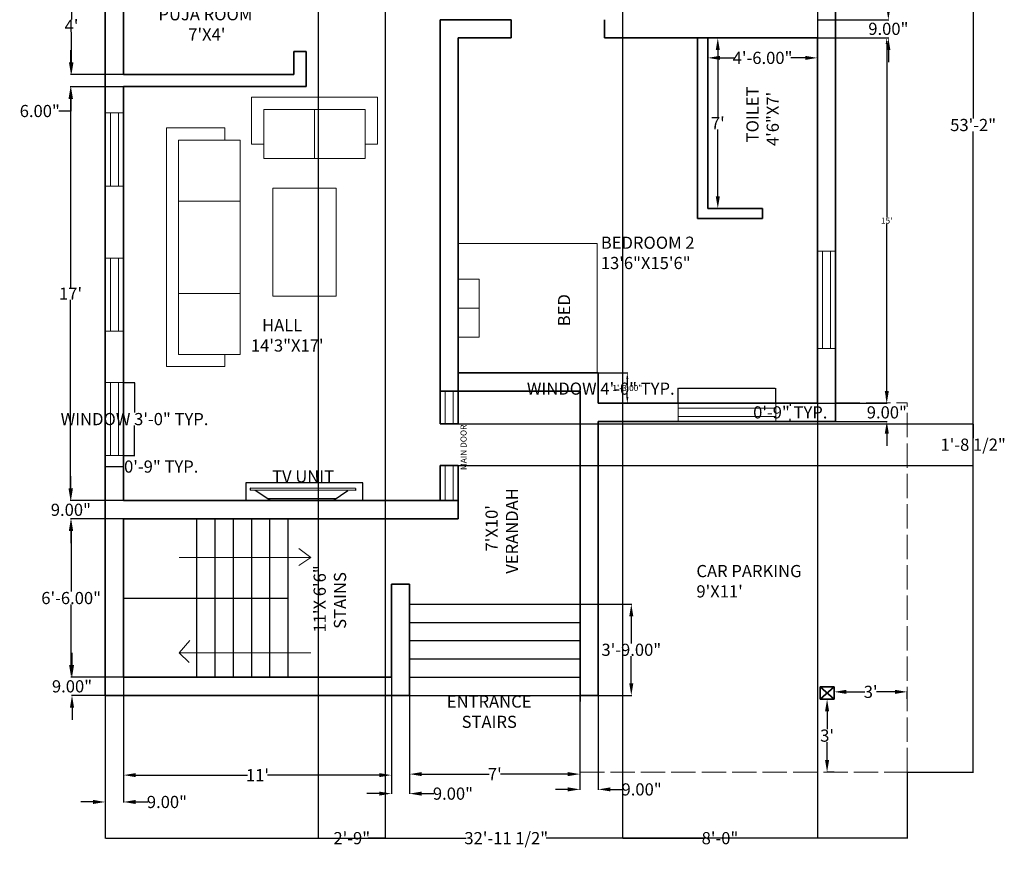
# Model space of a CAD drawing. Units: inches. Extents: x 14 to 1508, y -30 to 806.
# Tile 1 of 4: x 14 to 499, y 90 to 502. Entities that reach past the tile are written whole.
import ezdxf

# ---------------------------------------------------------------- set-up
doc = ezdxf.new("R2010")
doc.units = ezdxf.units.IN
doc.header["$MEASUREMENT"] = 0
doc.linetypes.add('ACAD_ISO02W100', pattern=[15, 12, -3])
for name, color, linetype, lineweight in [('A-ANNO-DIMS', 6, 'Continuous', 18), ('A-ANNO-SYMB', 2, 'Continuous', 18), ('A-ANNO-TEXT', 7, 'Continuous', 18), ('A-AREA-IDEN', 3, 'Continuous', 18), ('A-COLS', 7, 'Continuous', 35), ('A-FLOR-CASE', 8, 'Continuous', 25), ('A-FLOR-PRKG', 8, 'ACAD_ISO02W100', 18), ('A-FLOR-STRS', 7, 'Continuous', 25), ('A-FURN', 8, 'Continuous', 18), ('A-GLAZ', 4, 'Continuous', 18), ('A-WALL', 7, 'Continuous', 35)]:
    doc.layers.add(name, color=color, linetype=linetype, lineweight=lineweight)
doc.styles.get("Standard").update_dxf_attribs({"font": 'arial.ttf'})
doc.dimstyles.get("Standard").update_dxf_attribs({"dimtxt": 6, "dimasz": 0.18, "dimexe": 0.18, "dimexo": 0.0625, "dimgap": 0.09, "dimtad": 0, "dimtih": 1, "dimtoh": 1, "dimzin": 0, "dimdsep": 46, "dimlunit": 3, "dimtxsty": 'Standard', "dimcen": 0.09, "dimadec": 0, "dimazin": 0, "dimtfac": 1, "dimtofl": 0, "dimtmove": 0, "dimatfit": 3, "dimfxl": 1, "dimtolj": 1, "dimtzin": 0, "dimarcsym": 0})

# ---------------------------------------------------------------- blocks, each defined once
blk = doc.blocks.new('*D9')
at = {"layer": 'A-ANNO-DIMS', "color": 0, "lineweight": -2, "transparency": 16777216}
for p, q in [((64.9, 523.06), (39.11, 523.06)), ((39.29, 517.06), (39.29, 502.15)), ((39.29, 481.06), (39.29, 495.97)), ((64.9, 475.06), (39.11, 475.06))]:
    blk.add_line(p, q, dxfattribs=at)
at = {"layer": 'A-ANNO-DIMS', "color": 0, "transparency": 16777216}
for points in [[(38.29, 517.06), (40.29, 517.06), (39.29, 523.06)], [(38.29, 481.06), (40.29, 481.06), (39.29, 475.06)]]:
    blk.add_solid(points, dxfattribs=at)
at = {"layer": 'Defpoints', "color": 0, "transparency": 16777216}
for p in [(64.96, 523.06), (39.29, 475.06), (64.96, 475.06)]:
    blk.add_point(p, dxfattribs=at)
at = {"layer": 'A-ANNO-DIMS', "color": 0, "transparency": 16777216, "insert": (39.29, 499.06), "char_height": 6, "attachment_point": 5}
blk.add_mtext("\\A1;4'", dxfattribs=at)
blk = doc.blocks.new('*D10')
at = {"layer": 'A-ANNO-DIMS', "color": 0, "lineweight": -2, "transparency": 16777216}
for p, q in [((39.03, 481.06), (39.03, 487.06)), ((64.9, 475.06), (38.85, 475.06)), ((64.9, 469.06), (38.85, 469.06)), ((39.03, 463.06), (39.03, 457.06)), ((39.03, 457.06), (33.03, 457.06))]:
    blk.add_line(p, q, dxfattribs=at)
at = {"layer": 'A-ANNO-DIMS', "color": 0, "transparency": 16777216}
for points in [[(38.03, 481.06), (40.03, 481.06), (39.03, 475.06)], [(38.03, 463.06), (40.03, 463.06), (39.03, 469.06)]]:
    blk.add_solid(points, dxfattribs=at)
at = {"layer": 'Defpoints', "color": 0, "transparency": 16777216}
for p in [(64.96, 475.06), (39.03, 469.06), (64.96, 469.06)]:
    blk.add_point(p, dxfattribs=at)
at = {"layer": 'A-ANNO-DIMS', "color": 0, "transparency": 16777216, "insert": (23.65, 457.06), "char_height": 6, "attachment_point": 5}
blk.add_mtext('\\A1;6.00"', dxfattribs=at)
blk = doc.blocks.new('*D11')
at = {"layer": 'A-ANNO-DIMS', "color": 0, "lineweight": -2, "transparency": 16777216}
for p, q in [((64.9, 469.06), (38.64, 469.06)), ((38.82, 463.06), (38.82, 370.16)), ((38.82, 271.06), (38.82, 363.96)), ((64.9, 265.06), (38.64, 265.06))]:
    blk.add_line(p, q, dxfattribs=at)
at = {"layer": 'A-ANNO-DIMS', "color": 0, "transparency": 16777216}
for points in [[(37.82, 463.06), (39.82, 463.06), (38.82, 469.06)], [(37.82, 271.06), (39.82, 271.06), (38.82, 265.06)]]:
    blk.add_solid(points, dxfattribs=at)
at = {"layer": 'Defpoints', "color": 0, "transparency": 16777216}
for p in [(64.96, 469.06), (38.82, 265.06), (64.96, 265.06)]:
    blk.add_point(p, dxfattribs=at)
at = {"layer": 'A-ANNO-DIMS', "color": 0, "transparency": 16777216, "insert": (38.82, 367.06), "char_height": 6, "attachment_point": 5}
blk.add_mtext("\\A1;17'", dxfattribs=at)
blk = doc.blocks.new('*D12')
at = {"layer": 'A-ANNO-DIMS', "color": 0, "lineweight": -2, "transparency": 16777216}
for p, q in [((38.98, 271.06), (38.98, 277.06)), ((64.9, 265.06), (38.8, 265.06)), ((64.9, 256.06), (38.8, 256.06)), ((38.98, 250.06), (38.98, 244.06))]:
    blk.add_line(p, q, dxfattribs=at)
at = {"layer": 'A-ANNO-DIMS', "color": 0, "transparency": 16777216}
for points in [[(37.98, 271.06), (39.98, 271.06), (38.98, 265.06)], [(37.98, 250.06), (39.98, 250.06), (38.98, 256.06)]]:
    blk.add_solid(points, dxfattribs=at)
at = {"layer": 'Defpoints', "color": 0, "transparency": 16777216}
for p in [(64.96, 265.06), (38.98, 256.06), (64.96, 256.06)]:
    blk.add_point(p, dxfattribs=at)
at = {"layer": 'A-ANNO-DIMS', "color": 0, "transparency": 16777216, "insert": (38.98, 260.56), "char_height": 6, "attachment_point": 5}
blk.add_mtext('\\A1;9.00"', dxfattribs=at)
blk = doc.blocks.new('*D13')
at = {"layer": 'A-ANNO-DIMS', "color": 0, "lineweight": -2, "transparency": 16777216}
for p, q in [((64.9, 256.06), (38.94, 256.06)), ((39.12, 250.06), (39.12, 220.22)), ((39.12, 184.06), (39.12, 213.91)), ((64.9, 178.06), (38.94, 178.06))]:
    blk.add_line(p, q, dxfattribs=at)
at = {"layer": 'A-ANNO-DIMS', "color": 0, "transparency": 16777216}
for points in [[(38.12, 250.06), (40.12, 250.06), (39.12, 256.06)], [(38.12, 184.06), (40.12, 184.06), (39.12, 178.06)]]:
    blk.add_solid(points, dxfattribs=at)
at = {"layer": 'Defpoints', "color": 0, "transparency": 16777216}
for p in [(64.96, 256.06), (39.12, 178.06), (64.96, 178.06)]:
    blk.add_point(p, dxfattribs=at)
at = {"layer": 'A-ANNO-DIMS', "color": 0, "transparency": 16777216, "insert": (39.12, 217.06), "char_height": 6, "attachment_point": 5}
blk.add_mtext('\\A1;6\'-6.00"', dxfattribs=at)
blk = doc.blocks.new('*D14')
at = {"layer": 'A-ANNO-DIMS', "color": 0, "lineweight": -2, "transparency": 16777216}
for p, q in [((39.54, 184.06), (39.54, 190.06)), ((64.9, 178.06), (39.36, 178.06)), ((64.9, 169.06), (39.36, 169.06)), ((39.54, 163.06), (39.54, 157.06))]:
    blk.add_line(p, q, dxfattribs=at)
at = {"layer": 'A-ANNO-DIMS', "color": 0, "transparency": 16777216}
for points in [[(38.54, 184.06), (40.54, 184.06), (39.54, 178.06)], [(38.54, 163.06), (40.54, 163.06), (39.54, 169.06)]]:
    blk.add_solid(points, dxfattribs=at)
at = {"layer": 'Defpoints', "color": 0, "transparency": 16777216}
for p in [(64.96, 178.06), (39.54, 169.06), (64.96, 169.06)]:
    blk.add_point(p, dxfattribs=at)
at = {"layer": 'A-ANNO-DIMS', "color": 0, "transparency": 16777216, "insert": (39.54, 173.56), "char_height": 6, "attachment_point": 5}
blk.add_mtext('\\A1;9.00"', dxfattribs=at)
blk = doc.blocks.new('*D24')
at = {"layer": 'A-ANNO-DIMS', "color": 0, "lineweight": -2, "transparency": 16777216}
for p, q in [((441.97, 508.06), (441.97, 514.06)), ((407.03, 502.06), (442.15, 502.06)), ((407.03, 493.06), (442.15, 493.06)), ((441.97, 487.06), (441.97, 481.06))]:
    blk.add_line(p, q, dxfattribs=at)
at = {"layer": 'A-ANNO-DIMS', "color": 0, "transparency": 16777216}
for points in [[(440.97, 508.06), (442.97, 508.06), (441.97, 502.06)], [(440.97, 487.06), (442.97, 487.06), (441.97, 493.06)]]:
    blk.add_solid(points, dxfattribs=at)
at = {"layer": 'Defpoints', "color": 0, "transparency": 16777216}
for p in [(406.96, 502.06), (406.96, 493.06), (441.97, 493.06)]:
    blk.add_point(p, dxfattribs=at)
at = {"layer": 'A-ANNO-DIMS', "color": 0, "transparency": 16777216, "insert": (441.97, 497.56), "char_height": 6, "attachment_point": 5}
blk.add_mtext('\\A1;9.00"', dxfattribs=at)
blk = doc.blocks.new('*D25')
at = {"layer": 'A-ANNO-DIMS', "color": 0, "lineweight": -2, "transparency": 16777216}
for p, q in [((407.03, 493.06), (441.32, 493.06)), ((441.14, 490.06), (441.14, 404.68)), ((441.14, 316.06), (441.14, 401.44)), ((407.03, 313.06), (441.32, 313.06))]:
    blk.add_line(p, q, dxfattribs=at)
at = {"layer": 'A-ANNO-DIMS', "color": 0, "transparency": 16777216}
for points in [[(440.64, 490.06), (441.64, 490.06), (441.14, 493.06)], [(440.64, 316.06), (441.64, 316.06), (441.14, 313.06)]]:
    blk.add_solid(points, dxfattribs=at)
at = {"layer": 'Defpoints', "color": 0, "transparency": 16777216}
for p in [(406.96, 493.06), (406.96, 313.06), (441.14, 313.06)]:
    blk.add_point(p, dxfattribs=at)
at = {"layer": 'A-ANNO-DIMS', "color": 0, "transparency": 16777216, "insert": (441.14, 403.06), "char_height": 3, "attachment_point": 5}
blk.add_mtext("\\A1;15'", dxfattribs=at)
blk = doc.blocks.new('*D26')
at = {"layer": 'A-ANNO-DIMS', "color": 0, "lineweight": -2, "transparency": 16777216}
for p, q in [((441.21, 319.06), (441.21, 325.06)), ((407.03, 313.06), (441.39, 313.06)), ((407.03, 304.06), (441.39, 304.06)), ((441.21, 298.06), (441.21, 292.06))]:
    blk.add_line(p, q, dxfattribs=at)
at = {"layer": 'A-ANNO-DIMS', "color": 0, "transparency": 16777216}
for points in [[(440.21, 319.06), (442.21, 319.06), (441.21, 313.06)], [(440.21, 298.06), (442.21, 298.06), (441.21, 304.06)]]:
    blk.add_solid(points, dxfattribs=at)
at = {"layer": 'Defpoints', "color": 0, "transparency": 16777216}
for p in [(406.96, 313.06), (406.96, 304.06), (441.21, 304.06)]:
    blk.add_point(p, dxfattribs=at)
at = {"layer": 'A-ANNO-DIMS', "color": 0, "transparency": 16777216, "insert": (441.21, 308.56), "char_height": 6, "attachment_point": 5}
blk.add_mtext('\\A1;9.00"', dxfattribs=at)
blk = doc.blocks.new('*D28')
at = {"layer": 'A-ANNO-DIMS', "color": 0, "lineweight": -2, "transparency": 16777216}
for p, q in [((352.96, 493), (352.96, 483.07)), ((406.96, 493), (406.96, 483.07)), ((358.96, 483.25), (365.95, 483.25)), ((400.96, 483.25), (393.97, 483.25))]:
    blk.add_line(p, q, dxfattribs=at)
at = {"layer": 'A-ANNO-DIMS', "color": 0, "transparency": 16777216}
for points in [[(358.96, 484.25), (358.96, 482.25), (352.96, 483.25)], [(400.96, 484.25), (400.96, 482.25), (406.96, 483.25)]]:
    blk.add_solid(points, dxfattribs=at)
at = {"layer": 'Defpoints', "color": 0, "transparency": 16777216}
for p in [(352.96, 493.06), (406.96, 493.06), (406.96, 483.25)]:
    blk.add_point(p, dxfattribs=at)
at = {"layer": 'A-ANNO-DIMS', "color": 0, "transparency": 16777216, "insert": (379.96, 483.25), "char_height": 6, "attachment_point": 5}
blk.add_mtext('\\A1;4\'-6.00"', dxfattribs=at)
blk = doc.blocks.new('*D29')
at = {"layer": 'A-ANNO-DIMS', "color": 0, "lineweight": -2, "transparency": 16777216}
for p, q in [((353.03, 493.06), (358.07, 493.06)), ((357.89, 487.06), (357.89, 454.15)), ((357.89, 415.06), (357.89, 447.97)), ((353.03, 409.06), (358.07, 409.06))]:
    blk.add_line(p, q, dxfattribs=at)
at = {"layer": 'A-ANNO-DIMS', "color": 0, "transparency": 16777216}
for points in [[(356.89, 487.06), (358.89, 487.06), (357.89, 493.06)], [(356.89, 415.06), (358.89, 415.06), (357.89, 409.06)]]:
    blk.add_solid(points, dxfattribs=at)
at = {"layer": 'Defpoints', "color": 0, "transparency": 16777216}
for p in [(352.96, 493.06), (352.96, 409.06), (357.89, 409.06)]:
    blk.add_point(p, dxfattribs=at)
at = {"layer": 'A-ANNO-DIMS', "color": 0, "transparency": 16777216, "insert": (357.89, 451.06), "char_height": 6, "attachment_point": 5}
blk.add_mtext("\\A1;7'", dxfattribs=at)
blk = doc.blocks.new('*D30')
at = {"layer": 'A-ANNO-DIMS', "color": 0, "lineweight": -2, "transparency": 16777216}
for p, q in [((415.25, 167.32), (415.25, 171.01)), ((421.25, 170.83), (430.4, 170.83)), ((445.25, 170.83), (436.1, 170.83)), ((451.25, 167.32), (451.25, 171.01))]:
    blk.add_line(p, q, dxfattribs=at)
at = {"layer": 'A-ANNO-DIMS', "color": 0, "transparency": 16777216}
for points in [[(421.25, 171.83), (421.25, 169.83), (415.25, 170.83)], [(445.25, 171.83), (445.25, 169.83), (451.25, 170.83)]]:
    blk.add_solid(points, dxfattribs=at)
at = {"layer": 'Defpoints', "color": 0, "transparency": 16777216}
for p in [(451.25, 170.83), (415.25, 167.26), (451.25, 167.26)]:
    blk.add_point(p, dxfattribs=at)
at = {"layer": 'A-ANNO-DIMS', "color": 0, "transparency": 16777216, "insert": (433.25, 170.83), "char_height": 6, "attachment_point": 5}
blk.add_mtext("\\A1;3'", dxfattribs=at)
blk = doc.blocks.new('*D31')
at = {"layer": 'A-ANNO-DIMS', "color": 0, "lineweight": -2, "transparency": 16777216}
for p, q in [((415.19, 167.26), (411.59, 167.26)), ((411.77, 161.26), (411.77, 152.41)), ((411.77, 137.26), (411.77, 146.1)), ((415.19, 131.26), (411.59, 131.26))]:
    blk.add_line(p, q, dxfattribs=at)
at = {"layer": 'A-ANNO-DIMS', "color": 0, "transparency": 16777216}
for points in [[(410.77, 161.26), (412.77, 161.26), (411.77, 167.26)], [(410.77, 137.26), (412.77, 137.26), (411.77, 131.26)]]:
    blk.add_solid(points, dxfattribs=at)
at = {"layer": 'Defpoints', "color": 0, "transparency": 16777216}
for p in [(415.25, 167.26), (411.77, 131.26), (415.25, 131.26)]:
    blk.add_point(p, dxfattribs=at)
at = {"layer": 'A-ANNO-DIMS', "color": 0, "transparency": 16777216, "insert": (411.77, 149.26), "char_height": 6, "attachment_point": 5}
blk.add_mtext("\\A1;3'", dxfattribs=at)
blk = doc.blocks.new('*D32')
at = {"layer": 'A-ANNO-DIMS', "color": 0, "lineweight": -2, "transparency": 16777216}
for p, q in [((299.03, 214.06), (315.44, 214.06)), ((315.26, 208.06), (315.26, 194.72)), ((315.26, 175.06), (315.26, 188.41)), ((299.03, 169.06), (315.44, 169.06))]:
    blk.add_line(p, q, dxfattribs=at)
at = {"layer": 'A-ANNO-DIMS', "color": 0, "transparency": 16777216}
for points in [[(314.26, 208.06), (316.26, 208.06), (315.26, 214.06)], [(314.26, 175.06), (316.26, 175.06), (315.26, 169.06)]]:
    blk.add_solid(points, dxfattribs=at)
at = {"layer": 'Defpoints', "color": 0, "transparency": 16777216}
for p in [(298.96, 214.06), (298.96, 169.06), (315.26, 169.06)]:
    blk.add_point(p, dxfattribs=at)
at = {"layer": 'A-ANNO-DIMS', "color": 0, "transparency": 16777216, "insert": (315.26, 191.56), "char_height": 6, "attachment_point": 5}
blk.add_mtext('\\A1;3\'-9.00"', dxfattribs=at)
blk = doc.blocks.new('*D33')
at = {"layer": 'A-ANNO-DIMS', "color": 0, "lineweight": -2, "transparency": 16777216}
for p, q in [((299.03, 328.06), (313.47, 328.06)), ((313.29, 325.06), (313.29, 322.18)), ((313.29, 316.06), (313.29, 318.94)), ((299.03, 313.06), (313.47, 313.06))]:
    blk.add_line(p, q, dxfattribs=at)
at = {"layer": 'A-ANNO-DIMS', "color": 0, "transparency": 16777216}
for points in [[(312.79, 325.06), (313.79, 325.06), (313.29, 328.06)], [(312.79, 316.06), (313.79, 316.06), (313.29, 313.06)]]:
    blk.add_solid(points, dxfattribs=at)
at = {"layer": 'Defpoints', "color": 0, "transparency": 16777216}
for p in [(298.96, 328.06), (298.96, 313.06), (313.29, 313.06)]:
    blk.add_point(p, dxfattribs=at)
at = {"layer": 'A-ANNO-DIMS', "color": 0, "transparency": 16777216, "insert": (313.29, 320.56), "char_height": 3, "attachment_point": 5}
blk.add_mtext('\\A1;1\'-3.00"', dxfattribs=at)
blk = doc.blocks.new('*D34')
at = {"layer": 'A-ANNO-DIMS', "color": 0, "lineweight": -2, "transparency": 16777216}
for p, q in [((55.96, 178), (55.96, 116.39)), ((64.96, 178), (64.96, 116.39)), ((49.96, 116.57), (43.96, 116.57)), ((70.96, 116.57), (76.96, 116.57))]:
    blk.add_line(p, q, dxfattribs=at)
at = {"layer": 'A-ANNO-DIMS', "color": 0, "transparency": 16777216}
for points in [[(49.96, 117.57), (49.96, 115.57), (55.96, 116.57)], [(70.96, 117.57), (70.96, 115.57), (64.96, 116.57)]]:
    blk.add_solid(points, dxfattribs=at)
at = {"layer": 'Defpoints', "color": 0, "transparency": 16777216}
for p in [(55.96, 178.06), (64.96, 178.06), (64.96, 116.57)]:
    blk.add_point(p, dxfattribs=at)
at = {"layer": 'A-ANNO-DIMS', "color": 0, "transparency": 16777216, "insert": (86.33, 116.57), "char_height": 6, "attachment_point": 5}
blk.add_mtext('\\A1;9.00"', dxfattribs=at)
blk = doc.blocks.new('*D35')
at = {"layer": 'A-ANNO-DIMS', "color": 0, "lineweight": -2, "transparency": 16777216}
for p, q in [((64.96, 178), (64.96, 129.62)), ((196.96, 178), (196.96, 129.62)), ((70.96, 129.8), (126.06, 129.8)), ((190.96, 129.8), (135.86, 129.8))]:
    blk.add_line(p, q, dxfattribs=at)
at = {"layer": 'A-ANNO-DIMS', "color": 0, "transparency": 16777216}
for points in [[(70.96, 130.8), (70.96, 128.8), (64.96, 129.8)], [(190.96, 130.8), (190.96, 128.8), (196.96, 129.8)]]:
    blk.add_solid(points, dxfattribs=at)
at = {"layer": 'Defpoints', "color": 0, "transparency": 16777216}
for p in [(64.96, 178.06), (196.96, 178.06), (196.96, 129.8)]:
    blk.add_point(p, dxfattribs=at)
at = {"layer": 'A-ANNO-DIMS', "color": 0, "transparency": 16777216, "insert": (130.96, 129.8), "char_height": 6, "attachment_point": 5}
blk.add_mtext("\\A1;11'", dxfattribs=at)
blk = doc.blocks.new('*D36')
at = {"layer": 'A-ANNO-DIMS', "color": 0, "lineweight": -2, "transparency": 16777216}
for p, q in [((196.96, 169), (196.96, 120.5)), ((205.96, 169), (205.96, 120.5)), ((190.96, 120.68), (184.96, 120.68)), ((211.96, 120.68), (217.96, 120.68))]:
    blk.add_line(p, q, dxfattribs=at)
at = {"layer": 'A-ANNO-DIMS', "color": 0, "transparency": 16777216}
for points in [[(190.96, 121.68), (190.96, 119.68), (196.96, 120.68)], [(211.96, 121.68), (211.96, 119.68), (205.96, 120.68)]]:
    blk.add_solid(points, dxfattribs=at)
at = {"layer": 'Defpoints', "color": 0, "transparency": 16777216}
for p in [(196.96, 169.06), (205.96, 169.06), (205.96, 120.68)]:
    blk.add_point(p, dxfattribs=at)
at = {"layer": 'A-ANNO-DIMS', "color": 0, "transparency": 16777216, "insert": (227.33, 120.68), "char_height": 6, "attachment_point": 5}
blk.add_mtext('\\A1;9.00"', dxfattribs=at)
blk = doc.blocks.new('*D37')
at = {"layer": 'A-ANNO-DIMS', "color": 0, "lineweight": -2, "transparency": 16777216}
for p, q in [((205.96, 169), (205.96, 130.12)), ((289.96, 169), (289.96, 130.12)), ((211.96, 130.3), (245.14, 130.3)), ((283.96, 130.3), (250.79, 130.3))]:
    blk.add_line(p, q, dxfattribs=at)
at = {"layer": 'A-ANNO-DIMS', "color": 0, "transparency": 16777216}
for points in [[(211.96, 131.3), (211.96, 129.3), (205.96, 130.3)], [(283.96, 131.3), (283.96, 129.3), (289.96, 130.3)]]:
    blk.add_solid(points, dxfattribs=at)
at = {"layer": 'Defpoints', "color": 0, "transparency": 16777216}
for p in [(205.96, 169.06), (289.96, 169.06), (289.96, 130.3)]:
    blk.add_point(p, dxfattribs=at)
at = {"layer": 'A-ANNO-DIMS', "color": 0, "transparency": 16777216, "insert": (247.96, 130.3), "char_height": 6, "attachment_point": 5}
blk.add_mtext("\\A1;7'", dxfattribs=at)
blk = doc.blocks.new('*D38')
at = {"layer": 'A-ANNO-DIMS', "color": 0, "lineweight": -2, "transparency": 16777216}
for p, q in [((289.96, 169), (289.96, 122.59)), ((298.96, 169), (298.96, 122.59)), ((283.96, 122.77), (277.96, 122.77)), ((304.96, 122.77), (310.96, 122.77))]:
    blk.add_line(p, q, dxfattribs=at)
at = {"layer": 'A-ANNO-DIMS', "color": 0, "transparency": 16777216}
for points in [[(283.96, 123.77), (283.96, 121.77), (289.96, 122.77)], [(304.96, 123.77), (304.96, 121.77), (298.96, 122.77)]]:
    blk.add_solid(points, dxfattribs=at)
at = {"layer": 'Defpoints', "color": 0, "transparency": 16777216}
for p in [(289.96, 169.06), (298.96, 169.06), (298.96, 122.77)]:
    blk.add_point(p, dxfattribs=at)
at = {"layer": 'A-ANNO-DIMS', "color": 0, "transparency": 16777216, "insert": (320.33, 122.77), "char_height": 6, "attachment_point": 5}
blk.add_mtext('\\A1;9.00"', dxfattribs=at)
blk = doc.blocks.new('WIN-36IN')
for p, q in [((9, 36), (0, 36)), ((2.5, 36), (2.5, 0)), ((6.5, 36), (6.5, 0)), ((9, 0), (0, 0))]:
    blk.add_line(p, q)
blk.add_lwpolyline([(0, 36), (9, 36), (9, 0), (0, 0)], close=True)
blk = doc.blocks.new('WIN-48IN')
for p, q in [((0, 48), (9, 48)), ((2.5, 48), (2.5, 0)), ((6.5, 48), (6.5, 0)), ((0, 0), (9, 0))]:
    blk.add_line(p, q)
blk = doc.blocks.new('*D85')
at = {"layer": 'A-ANNO-DIMS', "color": 0, "lineweight": -2, "transparency": 16777216}
for p, q in [((65.03, 323.25), (70.54, 323.25)), ((70.36, 323.07), (70.36, 308.44)), ((70.36, 287.43), (70.36, 302.05)), ((65.03, 287.25), (70.54, 287.25))]:
    blk.add_line(p, q, dxfattribs=at)
at = {"layer": 'A-ANNO-DIMS', "color": 0, "transparency": 16777216}
for points in [[(70.33, 323.07), (70.39, 323.07), (70.36, 323.25)], [(70.33, 287.43), (70.39, 287.43), (70.36, 287.25)]]:
    blk.add_solid(points, dxfattribs=at)
at = {"layer": 'Defpoints', "color": 0, "transparency": 16777216}
for p in [(64.96, 323.25), (70.36, 323.25), (64.96, 287.25)]:
    blk.add_point(p, dxfattribs=at)
at = {"layer": 'A-ANNO-DIMS', "color": 0, "transparency": 16777216, "insert": (70.36, 305.25), "char_height": 6, "attachment_point": 5}
blk.add_mtext('\\A1;WINDOW 3\'-0" TYP.', dxfattribs=at)
blk = doc.blocks.new('*D86')
at = {"layer": 'A-ANNO-DIMS', "color": 0, "lineweight": -2, "transparency": 16777216}
for p, q in [((55.96, 287.18), (55.96, 281.67)), ((64.96, 287.18), (64.96, 281.67)), ((56.14, 281.85), (64.78, 281.85)), ((64.96, 281.85), (65.14, 281.85))]:
    blk.add_line(p, q, dxfattribs=at)
at = {"layer": 'A-ANNO-DIMS', "color": 0, "transparency": 16777216}
for points in [[(56.14, 281.88), (56.14, 281.82), (55.96, 281.85)], [(64.78, 281.88), (64.78, 281.82), (64.96, 281.85)]]:
    blk.add_solid(points, dxfattribs=at)
at = {"layer": 'Defpoints', "color": 0, "transparency": 16777216}
for p in [(55.96, 287.25), (64.96, 287.25), (64.96, 281.85)]:
    blk.add_point(p, dxfattribs=at)
at = {"layer": 'A-ANNO-DIMS', "color": 0, "transparency": 16777216, "insert": (83.52, 281.85), "char_height": 6, "attachment_point": 5}
blk.add_mtext('\\A1;0\'-9" TYP.', dxfattribs=at)
blk = doc.blocks.new('*D89')
at = {"layer": 'A-ANNO-DIMS', "color": 0, "lineweight": -2, "transparency": 16777216}
for p, q in [((338.42, 313.12), (338.42, 320.44)), ((386.42, 313.12), (386.42, 320.44)), ((338.42, 320.26), (338.24, 320.26)), ((386.24, 320.26), (338.6, 320.26))]:
    blk.add_line(p, q, dxfattribs=at)
at = {"layer": 'A-ANNO-DIMS', "color": 0, "transparency": 16777216}
for points in [[(338.6, 320.29), (338.6, 320.23), (338.42, 320.26)], [(386.24, 320.29), (386.24, 320.23), (386.42, 320.26)]]:
    blk.add_solid(points, dxfattribs=at)
at = {"layer": 'Defpoints', "color": 0, "transparency": 16777216}
for p in [(338.42, 320.26), (338.42, 313.06), (386.42, 313.06)]:
    blk.add_point(p, dxfattribs=at)
at = {"layer": 'A-ANNO-DIMS', "color": 0, "transparency": 16777216, "insert": (300.19, 320.26), "char_height": 6, "attachment_point": 5}
blk.add_mtext('\\A1;WINDOW 4\'-0" TYP.', dxfattribs=at)
blk = doc.blocks.new('*D90')
at = {"layer": 'A-ANNO-DIMS', "color": 0, "lineweight": -2, "transparency": 16777216}
for p, q in [((386.48, 313.06), (393.8, 313.06)), ((393.62, 312.88), (393.62, 311.72)), ((386.48, 304.06), (393.8, 304.06)), ((393.62, 304.24), (393.62, 305.41))]:
    blk.add_line(p, q, dxfattribs=at)
at = {"layer": 'A-ANNO-DIMS', "color": 0, "transparency": 16777216}
for points in [[(393.59, 312.88), (393.65, 312.88), (393.62, 313.06)], [(393.59, 304.24), (393.65, 304.24), (393.62, 304.06)]]:
    blk.add_solid(points, dxfattribs=at)
at = {"layer": 'Defpoints', "color": 0, "transparency": 16777216}
for p in [(386.42, 313.06), (393.62, 313.06), (386.42, 304.06)]:
    blk.add_point(p, dxfattribs=at)
at = {"layer": 'A-ANNO-DIMS', "color": 0, "transparency": 16777216, "insert": (393.62, 308.56), "char_height": 6, "attachment_point": 5}
blk.add_mtext('\\A1;0\'-9" TYP.', dxfattribs=at)
blk = doc.blocks.new('*D97')
at = {"layer": 'A-ANNO-DIMS', "color": 0, "lineweight": -2, "transparency": 16777216}
for p, q in [((55.96, 169), (55.96, 98.56)), ((451.25, 131.2), (451.25, 98.56)), ((56.14, 98.74), (233.89, 98.74)), ((451.07, 98.74), (273.32, 98.74))]:
    blk.add_line(p, q, dxfattribs=at)
at = {"layer": 'A-ANNO-DIMS', "color": 0, "transparency": 16777216}
for points in [[(56.14, 98.77), (56.14, 98.71), (55.96, 98.74)], [(451.07, 98.77), (451.07, 98.71), (451.25, 98.74)]]:
    blk.add_solid(points, dxfattribs=at)
at = {"layer": 'Defpoints', "color": 0, "transparency": 16777216}
for p in [(55.96, 169.06), (451.25, 131.26), (55.96, 98.74)]:
    blk.add_point(p, dxfattribs=at)
at = {"layer": 'A-ANNO-DIMS', "color": 0, "transparency": 16777216, "insert": (253.61, 98.74), "char_height": 6, "attachment_point": 5}
blk.add_mtext('\\A1;32\'-11 1/2"', dxfattribs=at)
blk = doc.blocks.new('*D99')
at = {"layer": 'A-ANNO-DIMS', "color": 0, "lineweight": -2, "transparency": 16777216}
for p, q in [((416.03, 769.06), (483.95, 769.06)), ((483.77, 768.88), (483.77, 453.32)), ((483.77, 131.44), (483.77, 447)), ((451.31, 131.26), (483.95, 131.26))]:
    blk.add_line(p, q, dxfattribs=at)
at = {"layer": 'A-ANNO-DIMS', "color": 0, "transparency": 16777216}
for points in [[(483.74, 768.88), (483.8, 768.88), (483.77, 769.06)], [(483.74, 131.44), (483.8, 131.44), (483.77, 131.26)]]:
    blk.add_solid(points, dxfattribs=at)
at = {"layer": 'Defpoints', "color": 0, "transparency": 16777216}
for p in [(415.96, 769.06), (483.77, 769.06), (451.25, 131.26)]:
    blk.add_point(p, dxfattribs=at)
at = {"layer": 'A-ANNO-DIMS', "color": 0, "transparency": 16777216, "insert": (483.77, 450.16), "char_height": 6, "attachment_point": 5}
blk.add_mtext('\\A1;53\'-2"', dxfattribs=at)
blk = doc.blocks.new('*D100')
at = {"layer": 'A-ANNO-DIMS', "color": 0, "lineweight": -2, "transparency": 16777216}
for p, q in [((160.96, 760), (160.96, 98.56)), ((193.96, 760), (193.96, 98.56)), ((161.14, 98.74), (169.35, 98.74)), ((193.78, 98.74), (185.58, 98.74))]:
    blk.add_line(p, q, dxfattribs=at)
at = {"layer": 'A-ANNO-DIMS', "color": 0, "transparency": 16777216}
for points in [[(161.14, 98.77), (161.14, 98.71), (160.96, 98.74)], [(193.78, 98.77), (193.78, 98.71), (193.96, 98.74)]]:
    blk.add_solid(points, dxfattribs=at)
at = {"layer": 'Defpoints', "color": 0, "transparency": 16777216}
for p in [(160.96, 760.06), (193.96, 760.06), (160.96, 98.74)]:
    blk.add_point(p, dxfattribs=at)
at = {"layer": 'A-ANNO-DIMS', "color": 0, "transparency": 16777216, "insert": (177.46, 98.74), "char_height": 6, "attachment_point": 5}
blk.add_mtext('\\A1;2\'-9"', dxfattribs=at)
blk = doc.blocks.new('*D101')
at = {"layer": 'A-ANNO-DIMS', "color": 0, "lineweight": -2, "transparency": 16777216}
for p, q in [((230.03, 302.87), (483.95, 302.87)), ((483.77, 302.69), (483.77, 295.82)), ((483.77, 282.56), (483.77, 289.43)), ((230.03, 282.38), (483.95, 282.38))]:
    blk.add_line(p, q, dxfattribs=at)
at = {"layer": 'A-ANNO-DIMS', "color": 0, "transparency": 16777216}
for points in [[(483.74, 302.69), (483.8, 302.69), (483.77, 302.87)], [(483.74, 282.56), (483.8, 282.56), (483.77, 282.38)]]:
    blk.add_solid(points, dxfattribs=at)
at = {"layer": 'Defpoints', "color": 0, "transparency": 16777216}
for p in [(229.96, 302.87), (483.77, 302.87), (229.96, 282.38)]:
    blk.add_point(p, dxfattribs=at)
at = {"layer": 'A-ANNO-DIMS', "color": 0, "transparency": 16777216, "insert": (483.77, 292.63), "char_height": 6, "attachment_point": 5}
blk.add_mtext('\\A1;1\'-8 1/2"', dxfattribs=at)
blk = doc.blocks.new('*D102')
at = {"layer": 'A-ANNO-DIMS', "color": 0, "lineweight": -2, "transparency": 16777216}
for p, q in [((310.96, 574), (310.96, 98.56)), ((406.96, 574), (406.96, 98.56)), ((311.14, 98.74), (350.89, 98.74)), ((406.78, 98.74), (367.03, 98.74))]:
    blk.add_line(p, q, dxfattribs=at)
at = {"layer": 'A-ANNO-DIMS', "color": 0, "transparency": 16777216}
for points in [[(311.14, 98.77), (311.14, 98.71), (310.96, 98.74)], [(406.78, 98.77), (406.78, 98.71), (406.96, 98.74)]]:
    blk.add_solid(points, dxfattribs=at)
at = {"layer": 'Defpoints', "color": 0, "transparency": 16777216}
for p in [(310.96, 574.06), (406.96, 574.06), (406.96, 98.74)]:
    blk.add_point(p, dxfattribs=at)
at = {"layer": 'A-ANNO-DIMS', "color": 0, "transparency": 16777216, "insert": (358.96, 98.74), "char_height": 6, "attachment_point": 5}
blk.add_mtext('\\A1;8\'-0"', dxfattribs=at)

msp = doc.modelspace()

# ---------------------------------------------------------------- linework, layer by layer
at = {"layer": 'A-ANNO-SYMB'}
for p, q in [((157.276, 237.035), (151.381, 241.478)), ((92.32, 237.035), (157.276, 237.035)), ((157.276, 237.035), (151.324, 233.112)), ((92.32, 190.08), (97.603, 196.171)), ((92.32, 190.08), (157.276, 190.08)), ((92.32, 190.08), (97.329, 185.352))]:
    msp.add_line(p, q, dxfattribs=at)
at = {"layer": 'A-COLS'}
for p, q in [((408.364, 173.302), (415.251, 167.258)), ((408.364, 167.258), (415.251, 173.302))]:
    msp.add_line(p, q, dxfattribs=at)
msp.add_lwpolyline([(408.364, 173.302), (415.251, 173.302), (415.251, 167.258), (408.364, 167.258)], close=True, dxfattribs=at)
at = {"layer": 'A-FLOR-CASE'}
for p, q in [((127.404, 271.242), (127.401, 270.242)), ((179.318, 270.065), (127.401, 270.242)), ((179.322, 271.065), (127.404, 271.242)), ((129.859, 270.234), (137.625, 265.062)), ((168.267, 265.062), (175.455, 270.078)), ((179.322, 271.065), (179.318, 270.065))]:
    msp.add_line(p, q, dxfattribs=at)
msp.add_lwpolyline([(125.193, 265.062), (182.834, 265.062), (182.834, 273.899), (125.193, 273.899)], close=True, dxfattribs=at)
msp.add_lwpolyline([(136.123, 266.062), (169.7, 266.062)], dxfattribs=at)
at = {"layer": 'A-FLOR-PRKG'}
for p, q in [((415.963, 313.198), (451.251, 313.198)), ((451.251, 131.258), (451.251, 313.198)), ((289.963, 166.062), (289.963, 131.258)), ((289.963, 131.258), (451.251, 131.258))]:
    msp.add_line(p, q, dxfattribs=at)
at = {"layer": 'A-FLOR-STRS'}
msp.add_line((64.963, 217.062), (145.963, 217.062), dxfattribs=at)
for points in [[(100.963, 256.062), (100.963, 178.062)], [(109.963, 256.062), (109.963, 178.062)], [(118.963, 256.062), (118.963, 178.062)], [(127.963, 256.062), (127.963, 178.062)], [(136.963, 256.062), (136.963, 178.062)], [(145.963, 256.062), (145.963, 178.062)], [(205.963, 214.062), (298.963, 214.062)], [(205.963, 205.062), (289.963, 205.062)], [(205.963, 196.062), (289.963, 196.062)], [(205.963, 187.062), (289.963, 187.062)], [(205.963, 178.062), (289.963, 178.062)], [(205.963, 169.062), (289.963, 169.062)]]:
    msp.add_lwpolyline(points, dxfattribs=at)
at = {"layer": 'A-FURN'}
for p, q in [((159.07, 433.731), (159.07, 457.889)), ((114.849, 442.714), (114.849, 448.714)), ((128.061, 440.673), (134.061, 440.673)), ((184.078, 440.673), (190.078, 440.673)), ((114.849, 331.139), (114.849, 337.139))]:
    msp.add_line(p, q, dxfattribs=at)
for points in [[(128.061, 440.673), (128.061, 463.889), (190.078, 463.889), (190.078, 440.673)], [(114.849, 331.139), (86.061, 331.139), (86.061, 448.714), (114.849, 448.714)], [(92.061, 441.533), (92.061, 442.714), (122.444, 442.714)], [(122.444, 442.714), (122.444, 337.139)], [(92.061, 337.139), (92.061, 441.533)], [(92.061, 412.714), (122.444, 412.714)], [(122.444, 367.139), (92.061, 367.139)], [(122.444, 337.139), (92.061, 337.139)]]:
    msp.add_lwpolyline(points, dxfattribs=at)
for points in [[(134.061, 457.889), (184.078, 457.889), (184.078, 433.731), (134.061, 433.731)], [(138.535, 419.042), (169.804, 419.042), (169.804, 365.781), (138.535, 365.781)], [(229.963, 328.062), (298.375, 328.062), (298.375, 391.832), (229.963, 391.832)], [(229.963, 359.947), (240.223, 359.947), (240.223, 374.21), (229.963, 374.21)], [(229.963, 359.947), (240.223, 359.947), (240.223, 345.684), (229.963, 345.684)]]:
    msp.add_lwpolyline(points, close=True, dxfattribs=at)
at = {"layer": 'A-GLAZ'}
for p, q in [((223.463, 302.871), (223.463, 319.062)), ((227.463, 302.871), (227.463, 319.062)), ((223.463, 282.382), (223.463, 265.062)), ((227.463, 282.382), (227.463, 265.062))]:
    msp.add_line(p, q, dxfattribs=at)
at = {"layer": 'A-WALL'}
for p, q in [((256.109, 502.062), (256.109, 493.062)), ((148.963, 486.398), (154.963, 486.398)), ((379.963, 409.062), (379.963, 404.062)), ((220.963, 302.871), (229.963, 302.871)), ((220.963, 282.382), (229.963, 282.382)), ((205.963, 223.903), (196.963, 223.903)), ((289.963, 169.062), (289.963, 166.062))]:
    msp.add_line(p, q, dxfattribs=at)
for points in [[(160.963, 769.062), (55.963, 769.062), (55.963, 169.062)], [(415.963, 304.062), (415.963, 769.062), (193.963, 769.062)], [(64.963, 523.062), (64.963, 475.062)], [(220.963, 502.062), (220.963, 469.062)], [(256.109, 502.062), (220.963, 502.062)], [(301.963, 493.062), (301.963, 502.062)], [(220.963, 302.871), (220.963, 493.062)], [(256.109, 493.062), (229.963, 493.062)], [(229.963, 302.871), (229.963, 493.062)], [(406.963, 493.062), (301.963, 493.062)], [(347.963, 404.062), (347.963, 493.062)], [(352.963, 409.062), (352.963, 493.062)], [(406.963, 313.062), (406.963, 493.062)], [(148.963, 486.398), (148.963, 475.062)], [(154.963, 486.398), (154.963, 469.062)], [(64.963, 475.062), (148.963, 475.062)], [(64.963, 469.062), (154.963, 469.062)], [(64.963, 469.062), (64.963, 265.062)], [(379.963, 409.062), (352.963, 409.062)], [(379.963, 404.062), (347.963, 404.062)], [(220.963, 328.062), (220.963, 319.062)], [(298.963, 328.062), (229.963, 328.062)], [(298.963, 313.062), (298.963, 328.062)], [(289.963, 319.062), (220.963, 319.062)], [(289.963, 169.062), (289.963, 319.062)], [(406.963, 313.062), (298.963, 313.062)], [(415.963, 304.062), (298.963, 304.062)], [(298.963, 169.062), (298.963, 304.062)], [(220.963, 265.062), (220.963, 282.382)], [(229.963, 256.062), (229.963, 282.382)], [(64.963, 265.062), (229.963, 265.062)], [(64.963, 256.062), (229.963, 256.062)], [(64.963, 256.062), (64.963, 178.062)], [(196.963, 223.903), (196.963, 178.062)], [(205.963, 223.903), (205.963, 169.062)], [(64.963, 178.062), (196.963, 178.062)], [(55.963, 169.062), (205.963, 169.062)], [(289.963, 169.062), (298.963, 169.062)]]:
    msp.add_lwpolyline(points, dxfattribs=at)

# ---------------------------------------------------------------- block references
at = {"layer": 'A-GLAZ'}
for name, p in [('WIN-36IN', (55.963, 420.102)), ('WIN-36IN', (55.963, 348.564)), ('WIN-48IN', (406.963, 339.957)), ('WIN-36IN', (55.963, 287.247))]:
    msp.add_blockref(name, p, dxfattribs=at)
at = {"layer": 'A-GLAZ', "rotation": 90.0000000000006}
msp.add_blockref('WIN-48IN', (386.422, 304.062), dxfattribs=at)

# ---------------------------------------------------------------- texts
at = {"layer": 'A-ANNO-TEXT', "attachment_point": 1, "rotation": 90}
for s, insert, char_height in [('BED', (279.105, 351), 6), ('MAIN DOOR', (231.054, 280.153), 3)]:
    msp.add_mtext_dynamic_manual_height_columns(s, width=241.93696, gutter_width=1, heights=[0], dxfattribs=dict(at, insert=insert, char_height=char_height))
at = {"layer": 'A-ANNO-TEXT', "insert": (138.179, 280.041), "char_height": 6, "attachment_point": 1}
msp.add_mtext_dynamic_manual_height_columns('TV UNIT', width=241.93696, gutter_width=1, heights=[0], dxfattribs=at)
at = {"layer": 'A-AREA-IDEN', "char_height": 6, "attachment_point": 1}
for s, insert in [("PUJA ROOM\\P        7'X4'", (82.167, 507.758)), ('BEDROOM 2\\P13\'6"X15\'6"', (300.226, 395.161)), ('             HALL\\P          14\'3"X17\'', (109.392, 354.501)), ("CAR PARKING\\P9'X11'", (347.342, 233.351)), ('ENTRANCE\\P    STAIRS', (224.288, 169.062))]:
    msp.add_mtext_dynamic_manual_height_columns(s, width=241.93696, gutter_width=1, heights=[0], dxfattribs=dict(at, insert=insert))
at = {"layer": 'A-AREA-IDEN', "char_height": 6, "attachment_point": 1, "rotation": 90}
for s, insert in [(' TOILET\\P4\'6"X7\'', (371.973, 439.786)), ("      7'X10'\\PVERANDAH", (243.398, 229.005)), ('  11\'X 6\'6"\\P   STAINS', (158.65, 196.397))]:
    msp.add_mtext_dynamic_manual_height_columns(s, width=241.93696, gutter_width=1, heights=[0], dxfattribs=dict(at, insert=insert))

# ---------------------------------------------------------------- dimensions: what is measured, and where the dimension line sits
at = {"layer": 'A-ANNO-DIMS'}
for base, p1, p2, override, picture, middle in [((483.766, 769.062), (451.251, 131.258), (415.963, 769.062), {"dimdec": 1, "dimlfac": 1, "dimrnd": 0, "dimzin": 1, "dimdsep": 46, "dimlunit": 4, "dimfrac": 2}, '*D99', (483.766, 450.16)), ((39.291, 475.062), (64.963, 523.062), (64.963, 475.062), {"dimasz": 6, "dimclrd": 0, "dimclre": 0, "dimclrt": 0}, '*D9', (39.291, 499.062)), ((441.972, 493.062), (406.963, 502.062), (406.963, 493.062), {"dimasz": 6, "dimclrd": 0, "dimclre": 0, "dimclrt": 0}, '*D24', (441.972, 497.562)), ((357.895, 409.062), (352.963, 493.062), (352.963, 409.062), {"dimasz": 6, "dimclrd": 0, "dimclre": 0, "dimclrt": 0}, '*D29', (357.895, 451.062)), ((441.142, 313.062), (406.963, 493.062), (406.963, 313.062), {"dimtxt": 3, "dimasz": 3, "dimclrd": 0, "dimclre": 0, "dimclrt": 0}, '*D25', (441.142, 403.062)), ((39.026, 469.062), (64.963, 475.062), (64.963, 469.062), {"dimasz": 6, "dimclrd": 0, "dimclre": 0, "dimclrt": 0}, '*D10', (23.645, 457.062)), ((38.822, 265.062), (64.963, 469.062), (64.963, 265.062), {"dimasz": 6, "dimclrd": 0, "dimclre": 0, "dimclrt": 0}, '*D11', (38.822, 367.062)), ((313.287, 313.062), (298.963, 328.062), (298.963, 313.062), {"dimtxt": 3, "dimasz": 3, "dimclrd": 0, "dimclre": 0, "dimclrt": 0}, '*D33', (313.287, 320.562)), ((441.208, 304.062), (406.963, 313.062), (406.963, 304.062), {"dimasz": 6, "dimclrd": 0, "dimclre": 0, "dimclrt": 0}, '*D26', (441.208, 308.562)), ((483.766, 302.871), (229.963, 282.382), (229.963, 302.871), {"dimdec": 1, "dimlfac": 1, "dimrnd": 0, "dimzin": 1, "dimdsep": 46, "dimlunit": 4, "dimfrac": 2}, '*D101', (483.766, 292.626)), ((38.976, 256.062), (64.963, 265.062), (64.963, 256.062), {"dimasz": 6, "dimclrd": 0, "dimclre": 0, "dimclrt": 0}, '*D12', (38.976, 260.562)), ((39.116, 178.062), (64.963, 256.062), (64.963, 178.062), {"dimasz": 6, "dimclrd": 0, "dimclre": 0, "dimclrt": 0}, '*D13', (39.116, 217.062)), ((315.263, 169.062), (298.963, 214.062), (298.963, 169.062), {"dimasz": 6, "dimclrd": 0, "dimclre": 0, "dimclrt": 0}, '*D32', (315.263, 191.562)), ((39.545, 169.062), (64.963, 178.062), (64.963, 169.062), {"dimasz": 6, "dimclrd": 0, "dimclre": 0, "dimclrt": 0}, '*D14', (39.545, 173.562)), ((411.768, 131.258), (415.251, 167.258), (415.251, 131.258), {"dimasz": 6, "dimclrd": 0, "dimclre": 0, "dimclrt": 0}, '*D31', (411.768, 149.258))]:
    dim = msp.add_linear_dim(base=base, p1=p1, p2=p2, angle=90, dimstyle='Standard', override=override, dxfattribs=at)
    dim.commit()
    dim.dimension.update_dxf_attribs({"geometry": picture, "text_midpoint": middle})
for base, p1, p2, override, picture, middle in [((160.963, 98.743), (193.963, 760.062), (160.963, 760.062), {"dimdec": 1, "dimlfac": 1, "dimrnd": 0, "dimzin": 1, "dimdsep": 46, "dimlunit": 4, "dimfrac": 2}, '*D100', (177.463, 98.743)), ((406.963, 98.743), (310.963, 574.062), (406.963, 574.062), {"dimdec": 1, "dimlfac": 1, "dimrnd": 0, "dimzin": 1, "dimdsep": 46, "dimlunit": 4, "dimfrac": 2}, '*D102', (358.963, 98.743)), ((406.963, 483.245), (352.963, 493.062), (406.963, 493.062), {"dimasz": 6, "dimclrd": 0, "dimclre": 0, "dimclrt": 0}, '*D28', (379.963, 483.245)), ((64.963, 116.57), (55.963, 178.062), (64.963, 178.062), {"dimasz": 6, "dimclrd": 0, "dimclre": 0, "dimclrt": 0}, '*D34', (86.327, 116.57)), ((196.963, 129.8), (64.963, 178.062), (196.963, 178.062), {"dimasz": 6, "dimclrd": 0, "dimclre": 0, "dimclrt": 0}, '*D35', (130.963, 129.8)), ((451.251, 170.826), (415.251, 167.258), (451.251, 167.258), {"dimasz": 6, "dimclrd": 0, "dimclre": 0, "dimclrt": 0}, '*D30', (433.251, 170.826)), ((55.963, 98.743), (451.251, 131.258), (55.963, 169.062), {"dimdec": 1, "dimlfac": 1, "dimrnd": 0, "dimzin": 1, "dimdsep": 46, "dimlunit": 4, "dimfrac": 2}, '*D97', (253.607, 98.743)), ((205.963, 120.676), (196.963, 169.062), (205.963, 169.062), {"dimasz": 6, "dimclrd": 0, "dimclre": 0, "dimclrt": 0}, '*D36', (227.327, 120.676)), ((289.963, 130.297), (205.963, 169.062), (289.963, 169.062), {"dimasz": 6, "dimclrd": 0, "dimclre": 0, "dimclrt": 0}, '*D37', (247.963, 130.297)), ((298.963, 122.768), (289.963, 169.062), (298.963, 169.062), {"dimasz": 6, "dimclrd": 0, "dimclre": 0, "dimclrt": 0}, '*D38', (320.327, 122.768))]:
    dim = msp.add_linear_dim(base=base, p1=p1, p2=p2, dimstyle='Standard', override=override, dxfattribs=at)
    dim.commit()
    dim.dimension.update_dxf_attribs({"geometry": picture, "text_midpoint": middle})
for base, p1, p2, angle, text, picture, middle in [((338.422, 320.262), (386.422, 313.062), (338.422, 313.062), 180, 'WINDOW <> TYP.', '*D89', (300.19, 320.262)), ((70.363, 323.247), (64.963, 287.247), (64.963, 323.247), 90, 'WINDOW <> TYP.', '*D85', (70.363, 305.247)), ((393.622, 313.062), (386.422, 304.062), (386.422, 313.062), 90, '<> TYP.', '*D90', (393.622, 308.562))]:
    dim = msp.add_linear_dim(base=base, p1=p1, p2=p2, angle=angle, text=text, dimstyle='Standard', override={"dimdec": 1, "dimlfac": 1, "dimrnd": 0, "dimzin": 1, "dimdsep": 46, "dimlunit": 4, "dimfrac": 2}, dxfattribs=at)
    dim.commit()
    dim.dimension.update_dxf_attribs({"geometry": picture, "text_midpoint": middle})
dim = msp.add_linear_dim(base=(64.963, 281.847), p1=(55.963, 287.247), p2=(64.963, 287.247), text='<> TYP.', dimstyle='Standard', override={"dimdec": 1, "dimlfac": 1, "dimrnd": 0, "dimzin": 1, "dimdsep": 46, "dimlunit": 4, "dimfrac": 2}, dxfattribs=at)
dim.commit()
dim.dimension.update_dxf_attribs({"geometry": '*D86', "text_midpoint": (83.519, 281.847)})

doc.saveas('drawing.dxf')
